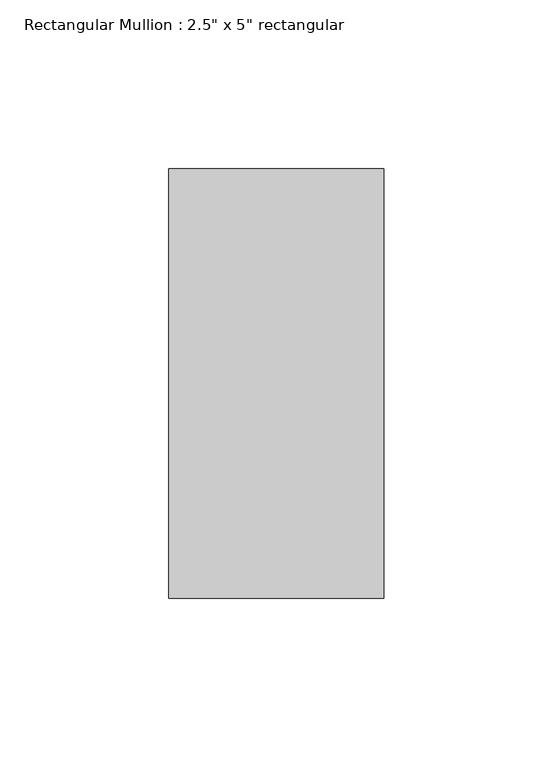
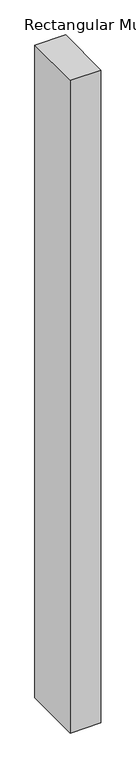
"""IFC4 building model written with IfcOpenShell, lengths in millimetres: member geometry."""

from ifc_helpers import new_model, si_unit, frame, origin, place, context, project, spatial, polyline, outline, extrude, source, transform, mapped, element, save


def member_e39930a5(model_context):
    return source(origin(), model_context, "Body", "SweptSolid", [
        extrude(outline(polyline([(0.0, 63.5), (0.0, -63.5), (-63.5, -63.5), (-63.5, 63.5), (0.0, 63.5)])), frame((0.0, 0.0, -1432.2179754), z_axis=(0.0, 0.0, 1.0), x_axis=(1.0, 0.0, 0.0)), (0.0, 0.0, 1.0), 1432.2179754),
    ])


if __name__ == "__main__":
    model = new_model("IFC4")
    model_context = context("Model", 3, world=origin())
    ifc_project = project(units=[si_unit("LENGTHUNIT", "METRE", prefix="MILLI")], contexts=[model_context])
    site = spatial("IfcSite", under=ifc_project)
    building = spatial("IfcBuilding", under=site)
    placement = place(None, origin())
    member_shape = member_e39930a5(model_context)
    element("IfcMember", 1, ObjectType="Rectangular Mullion : 2.5\" x 5\" rectangular", at=placement, inside=building, context=model_context, shape_type="MappedRepresentation", body=[
        mapped(member_shape, transform((0.0, 0.0, 0.0), x_axis=(1.0, 0.0, 0.0), y_axis=(0.0, 1.0, 0.0), z_axis=(0.0, 0.0, 1.0))),
    ])
    save(model, "model.ifc")

# Revit data of these elements
# Type "Rectangular Mullion : 2.5\" x 5\" rectangular"
#   built-in parameter 1007304 = 0.416667 (stored number, unit not read)
#   built-in parameter 1007301 = 0.104167 (stored number, unit not read)
#   built-in parameter 1007300 = 0.104167 (stored number, unit not read)
# Element 1 (IfcMember, "Rectangular Mullion : 2.5\" x 5\" rectangular")
#   Materials on its faces: "Aluminum"
# Materials
#   "Aluminum": class "Metal", colour RGB 247 247 247, transparency 0, Description = "Aluminum 6061", Cost = 0
